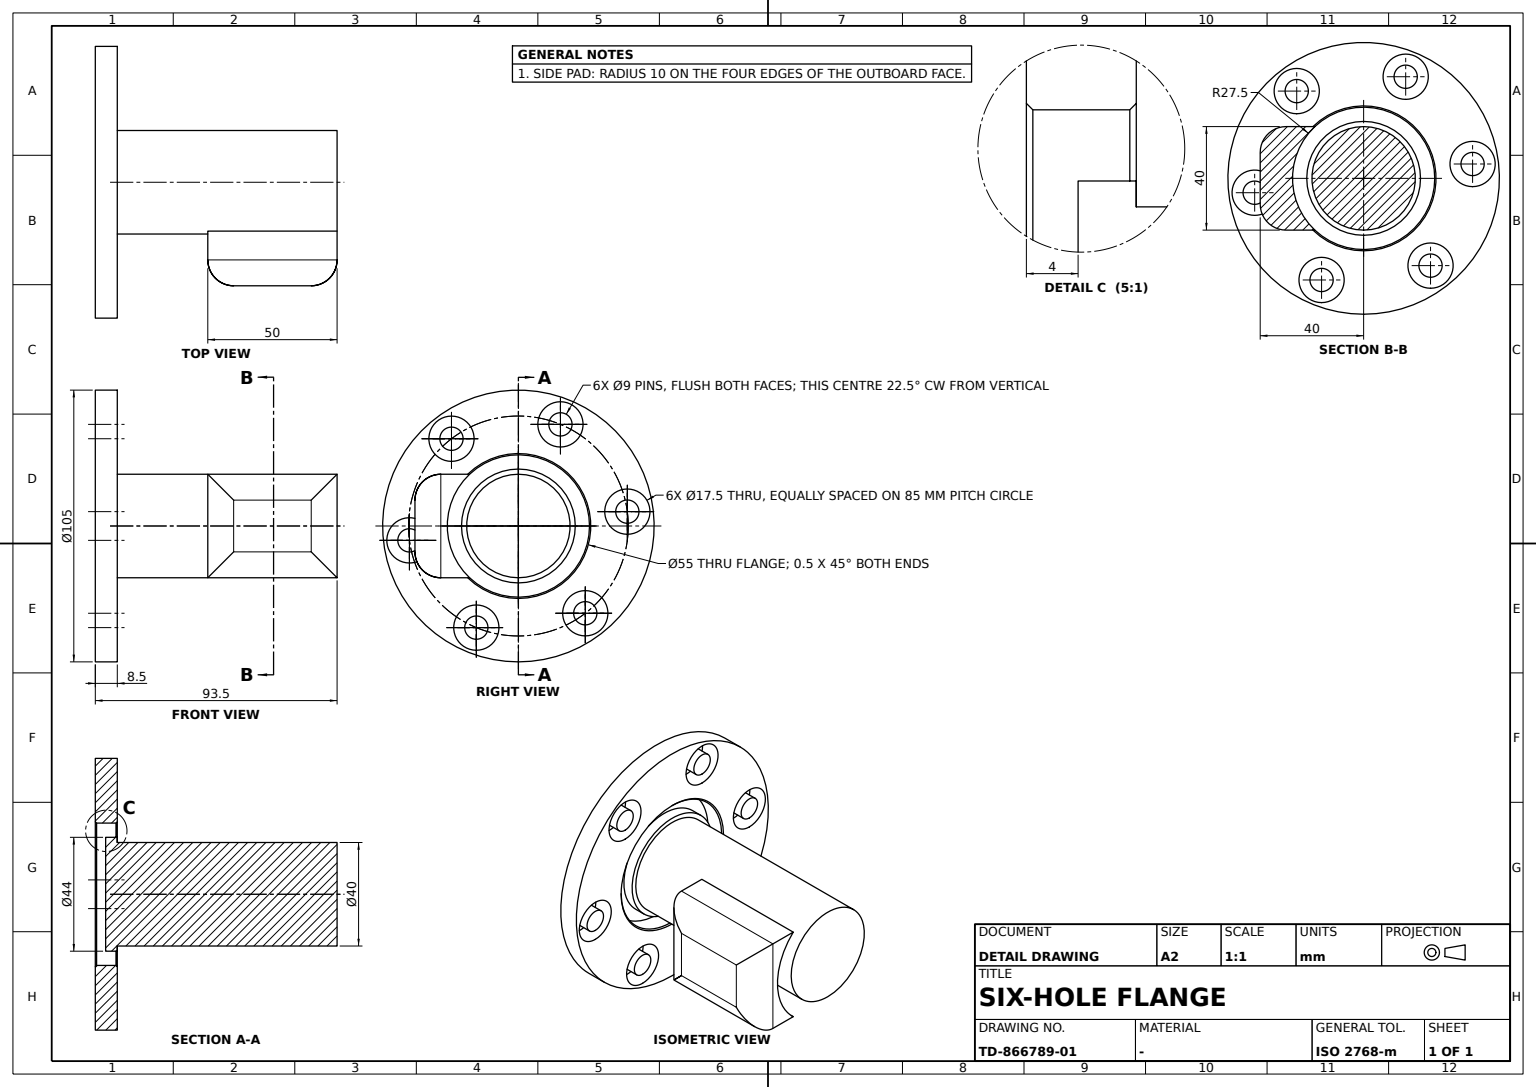
CATIA V5 part; units mm, degrees
sketch "Sketch1" plane through (0, 0, 0) normal (0, 0, 1) x (1, 0, 0)
  circle A0 centre (0, 0) radius 52.5
  line L0 (-90, 0) -> (120, 0) construction
  point P0 (-90, 0)
  line L1 (0, 0) -> (-92.388, 38.2683) construction
  circle A1 centre (-39.2649, 16.264) radius 8.75
  point P1 (-39.2649, 16.264)
  circle A2 centre (-39.2649, 16.264) radius 4.5
  circle A3 centre (-33.7175, -25.8724) radius 8.75
  circle A4 centre (-33.7175, -25.8724) radius 4.5
  circle A5 centre (5.5474, -42.1364) radius 8.75
  circle A6 centre (5.5474, -42.1364) radius 4.5
  circle A7 centre (39.2649, -16.264) radius 8.75
  circle A8 centre (39.2649, -16.264) radius 4.5
  circle A9 centre (33.7175, 25.8724) radius 8.75
  circle A10 centre (33.7175, 25.8724) radius 4.5
  circle A11 centre (-5.5474, 42.1364) radius 8.75
  circle A12 centre (-5.5474, 42.1364) radius 4.5
  circle A13 centre (0, 0) radius 27.5
  circle A14 centre (0, 0) radius 22
  dimension "radius A0" = 52.5
  dimension "angle L1 L0" = 22.5
  dimension "distance P1 origin" = 42.5
  dimension "radius A1" = 8.75
  dimension "radius A2" = 4.5
  dimension "radius A13" = 27.5
  dimension "radius A14" = 22
  constraint coincidence P0 x-axis
  constraint coincidence P1 L1
  constraint horizontal L0 x-axis
extrude "Pad1" add sketch "Sketch1" along normal blind 8.5
sketch "Sketch2" plane through (0, 0, 8.5) normal (0, 0, 1) x (1, 0, 0)
  circle A0 centre (0, 0) radius 20
extrude "Pad2" add sketch "Sketch2" along normal blind 85
sketch "Sketch3" plane through (0, 0, 93.5) normal (0, 0, 1) x (1, 0, 0)
  line L0 (20, -18.8746) -> (20, -40)
  line L1 (20, -40) -> (-20, -40)
  line L2 (-20, -40) -> (-20, -18.8746)
  arc A0 (-20, -18.8746) -> (20, -18.8746) centre (0, 0) ccw
  circle A1 centre (0, 0) radius 27.5 construction
  dimension "length L1" = 40
  dimension "distance x axis L1" = 40
  constraint vertical L0 y-axis
  constraint vertical L2 y-axis
  constraint horizontal L1 x-axis
  constraint equidistance L0 L2 origin
  constraint coincidence A0 A1
extrude "Pad3" add sketch "Sketch3" against normal blind 50
sketch "Sketch4" plane through (18.3835, 34.4905, 0) normal (0, 0, -1) x (1, 0, 0)
  point P0 (-20, 34.4905)
hole "Hole1" at (-1.6165, 0, 0) direction (0, 0, 1) diameter 50 depth 4
chamfer "Chamfer1" distance 0.5 angle 45 2 edges at (-27.5, 0, 0) (-27.5, 0, 8.5)
fillet "Fillet1" radius 10 4 edges at (0, -40, 93.5) (20, -40, 68.5) (-20, -40, 68.5) (0, -40, 43.5)
